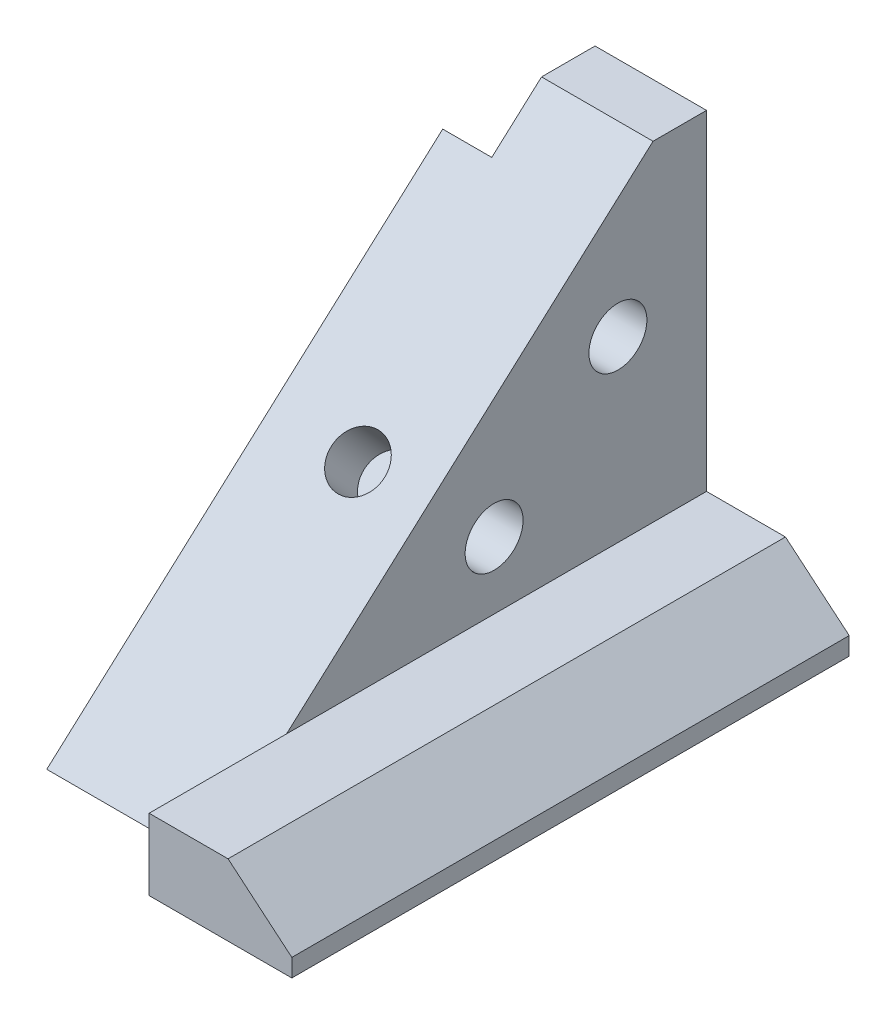
ISO-10303-21;
HEADER;
FILE_DESCRIPTION(('STEP AP214'),'2;1');
FILE_NAME('part.step','',(''),(''),'','','');
FILE_SCHEMA(('AUTOMOTIVE_DESIGN { 1 0 10303 214 1 1 1 1 }'));
ENDSEC;
DATA;
#1=APPLICATION_CONTEXT('core data for automotive mechanical design processes');
#2=APPLICATION_PROTOCOL_DEFINITION('international standard','automotive_design',2000,#1);
#3=PRODUCT_CONTEXT('',#1,'mechanical');
#4=PRODUCT('Part','Part','',(#3));
#5=PRODUCT_RELATED_PRODUCT_CATEGORY('part','',(#4));
#6=PRODUCT_DEFINITION_FORMATION('','',#4);
#7=PRODUCT_DEFINITION_CONTEXT('part definition',#1,'design');
#8=PRODUCT_DEFINITION('design','',#6,#7);
#9=PRODUCT_DEFINITION_SHAPE('','',#8);
#10=(LENGTH_UNIT() NAMED_UNIT(*) SI_UNIT(.MILLI.,.METRE.));
#11=(NAMED_UNIT(*) PLANE_ANGLE_UNIT() SI_UNIT($,.RADIAN.));
#12=(NAMED_UNIT(*) SI_UNIT($,.STERADIAN.) SOLID_ANGLE_UNIT());
#13=UNCERTAINTY_MEASURE_WITH_UNIT(LENGTH_MEASURE(1.E-05),#10,'distance_accuracy_value','');
#14=(GEOMETRIC_REPRESENTATION_CONTEXT(3) GLOBAL_UNCERTAINTY_ASSIGNED_CONTEXT((#13)) GLOBAL_UNIT_ASSIGNED_CONTEXT((#10,
#11,#12)) REPRESENTATION_CONTEXT('',''));
#15=CARTESIAN_POINT('',(0.,0.,0.));
#16=DIRECTION('',(0.,0.,1.));
#17=DIRECTION('',(1.,0.,0.));
#18=AXIS2_PLACEMENT_3D('',#15,#16,#17);
#19=CARTESIAN_POINT('',(0.,0.,125.));
#20=DIRECTION('',(0.,0.,1.));
#21=DIRECTION('',(1.,0.,0.));
#22=AXIS2_PLACEMENT_3D('',#19,#20,#21);
#23=PLANE('',#22);
#24=DIRECTION('',(-1.,0.,0.));
#25=VECTOR('',#24,1.);
#26=CARTESIAN_POINT('',(0.,16.,125.));
#27=LINE('',#26,#25);
#28=CARTESIAN_POINT('',(17.6989568888694,16.,125.));
#29=VERTEX_POINT('',#28);
#30=CARTESIAN_POINT('',(0.,16.,125.));
#31=VERTEX_POINT('',#30);
#32=EDGE_CURVE('E148',#29,#31,#27,.T.);
#33=ORIENTED_EDGE('',*,*,#32,.T.);
#34=DIRECTION('',(0.,1.,0.));
#35=VECTOR('',#34,1.);
#36=CARTESIAN_POINT('',(0.,90.,125.));
#37=LINE('',#36,#35);
#38=CARTESIAN_POINT('',(0.,0.,125.));
#39=VERTEX_POINT('',#38);
#40=EDGE_CURVE('E199',#39,#31,#37,.T.);
#41=ORIENTED_EDGE('',*,*,#40,.F.);
#42=DIRECTION('',(-1.,0.,0.));
#43=VECTOR('',#42,1.);
#44=CARTESIAN_POINT('',(0.,0.,125.));
#45=LINE('',#44,#43);
#46=CARTESIAN_POINT('',(32.,0.,125.));
#47=VERTEX_POINT('',#46);
#48=EDGE_CURVE('E164',#47,#39,#45,.T.);
#49=ORIENTED_EDGE('',*,*,#48,.F.);
#50=DIRECTION('',(0.,1.,0.));
#51=VECTOR('',#50,1.);
#52=CARTESIAN_POINT('',(32.,0.,125.));
#53=LINE('',#52,#51);
#54=CARTESIAN_POINT('',(32.,4.,125.));
#55=VERTEX_POINT('',#54);
#56=EDGE_CURVE('E210',#47,#55,#53,.T.);
#57=ORIENTED_EDGE('',*,*,#56,.T.);
#58=DIRECTION('',(-0.766044443118979,0.642787609686538,0.));
#59=VECTOR('',#58,1.);
#60=CARTESIAN_POINT('',(15.1912446633535,18.1042204035292,125.));
#61=LINE('',#60,#59);
#62=EDGE_CURVE('E206',#55,#29,#61,.T.);
#63=ORIENTED_EDGE('',*,*,#62,.T.);
#64=EDGE_LOOP('',(#33,#41,#49,#57,#63));
#65=FACE_BOUND('',#64,.T.);
#66=ADVANCED_FACE('F41',(#65),#23,.T.);
#67=CARTESIAN_POINT('',(-36.,0.,125.));
#68=DIRECTION('',(-1.,0.,0.));
#69=DIRECTION('',(0.,0.,1.));
#70=AXIS2_PLACEMENT_3D('',#67,#68,#69);
#71=PLANE('',#70);
#72=CARTESIAN_POINT('',(-36.,56.,19.8712945069006));
#73=DIRECTION('',(-1.,0.,0.));
#74=DIRECTION('',(0.,0.,1.));
#75=AXIS2_PLACEMENT_3D('',#72,#73,#74);
#76=CIRCLE('',#75,6.5);
#77=CARTESIAN_POINT('',(-36.,56.,26.3712945069006));
#78=VERTEX_POINT('',#77);
#79=EDGE_CURVE('E407',#78,#78,#76,.T.);
#80=ORIENTED_EDGE('',*,*,#79,.F.);
#81=EDGE_LOOP('',(#80));
#82=FACE_BOUND('',#81,.T.);
#83=CARTESIAN_POINT('',(-36.,31.,47.6366073776308));
#84=DIRECTION('',(-1.,0.,0.));
#85=DIRECTION('',(0.,0.,1.));
#86=AXIS2_PLACEMENT_3D('',#83,#84,#85);
#87=CIRCLE('',#86,6.5);
#88=CARTESIAN_POINT('',(-36.,31.,54.1366073776308));
#89=VERTEX_POINT('',#88);
#90=EDGE_CURVE('E398',#89,#89,#87,.T.);
#91=ORIENTED_EDGE('',*,*,#90,.F.);
#92=EDGE_LOOP('',(#91));
#93=FACE_BOUND('',#92,.T.);
#94=DIRECTION('',(0.,0.707106781186555,0.70710678118654));
#95=VECTOR('',#94,1.);
#96=CARTESIAN_POINT('',(-36.,51.1182175936227,-5.66857897078022));
#97=LINE('',#96,#95);
#98=CARTESIAN_POINT('',(-36.,56.7867965644031,0.));
#99=VERTEX_POINT('',#98);
#100=CARTESIAN_POINT('',(-36.,79.9492667239713,23.1624701595678));
#101=VERTEX_POINT('',#100);
#102=EDGE_CURVE('E124',#99,#101,#97,.T.);
#103=ORIENTED_EDGE('',*,*,#102,.F.);
#104=DIRECTION('',(0.,1.,0.));
#105=VECTOR('',#104,1.);
#106=CARTESIAN_POINT('',(-36.,0.,0.));
#107=LINE('',#106,#105);
#108=CARTESIAN_POINT('',(-36.,0.,0.));
#109=VERTEX_POINT('',#108);
#110=EDGE_CURVE('E133',#109,#99,#107,.T.);
#111=ORIENTED_EDGE('',*,*,#110,.F.);
#112=DIRECTION('',(0.,0.,-1.));
#113=VECTOR('',#112,1.);
#114=CARTESIAN_POINT('',(-36.,0.,125.));
#115=LINE('',#114,#113);
#116=CARTESIAN_POINT('',(-36.,0.,111.955126334629));
#117=VERTEX_POINT('',#116);
#118=EDGE_CURVE('E177',#117,#109,#115,.T.);
#119=ORIENTED_EDGE('',*,*,#118,.F.);
#120=DIRECTION('',(0.,-0.669130606358854,0.743144825477398));
#121=VECTOR('',#120,1.);
#122=CARTESIAN_POINT('',(-36.,90.,12.));
#123=LINE('',#122,#121);
#124=EDGE_CURVE('E130',#101,#117,#123,.T.);
#125=ORIENTED_EDGE('',*,*,#124,.F.);
#126=EDGE_LOOP('',(#103,#111,#119,#125));
#127=FACE_BOUND('',#126,.T.);
#128=ADVANCED_FACE('F43',(#82,#93,#127),#71,.T.);
#129=CARTESIAN_POINT('',(0.,0.,125.));
#130=DIRECTION('',(0.,-1.,0.));
#131=DIRECTION('',(1.,0.,0.));
#132=AXIS2_PLACEMENT_3D('',#129,#130,#131);
#133=PLANE('',#132);
#134=DIRECTION('',(-1.,0.,0.));
#135=VECTOR('',#134,1.);
#136=CARTESIAN_POINT('',(0.,0.,111.955126334629));
#137=LINE('',#136,#135);
#138=CARTESIAN_POINT('',(0.,0.,111.955126334629));
#139=VERTEX_POINT('',#138);
#140=EDGE_CURVE('E145',#139,#117,#137,.T.);
#141=ORIENTED_EDGE('',*,*,#140,.T.);
#142=ORIENTED_EDGE('',*,*,#118,.T.);
#143=DIRECTION('',(-1.,0.,0.));
#144=VECTOR('',#143,1.);
#145=CARTESIAN_POINT('',(0.,0.,0.));
#146=LINE('',#145,#144);
#147=CARTESIAN_POINT('',(32.,0.,0.));
#148=VERTEX_POINT('',#147);
#149=EDGE_CURVE('E142',#148,#109,#146,.T.);
#150=ORIENTED_EDGE('',*,*,#149,.F.);
#151=DIRECTION('',(0.,0.,-1.));
#152=VECTOR('',#151,1.);
#153=CARTESIAN_POINT('',(32.,0.,125.));
#154=LINE('',#153,#152);
#155=EDGE_CURVE('E180',#47,#148,#154,.T.);
#156=ORIENTED_EDGE('',*,*,#155,.F.);
#157=ORIENTED_EDGE('',*,*,#48,.T.);
#158=DIRECTION('',(0.,0.,1.));
#159=VECTOR('',#158,1.);
#160=CARTESIAN_POINT('',(0.,0.,111.955126334629));
#161=LINE('',#160,#159);
#162=EDGE_CURVE('E61',#139,#39,#161,.T.);
#163=ORIENTED_EDGE('',*,*,#162,.F.);
#164=EDGE_LOOP('',(#141,#142,#150,#156,#157,#163));
#165=FACE_BOUND('',#164,.T.);
#166=ADVANCED_FACE('F234',(#165),#133,.T.);
#167=CARTESIAN_POINT('',(32.,0.,125.));
#168=DIRECTION('',(-1.,0.,0.));
#169=DIRECTION('',(0.,0.,1.));
#170=AXIS2_PLACEMENT_3D('',#167,#168,#169);
#171=PLANE('',#170);
#172=DIRECTION('',(0.,1.,0.));
#173=VECTOR('',#172,1.);
#174=CARTESIAN_POINT('',(32.,0.,0.));
#175=LINE('',#174,#173);
#176=CARTESIAN_POINT('',(32.,4.,0.));
#177=VERTEX_POINT('',#176);
#178=EDGE_CURVE('E144',#148,#177,#175,.T.);
#179=ORIENTED_EDGE('',*,*,#178,.T.);
#180=DIRECTION('',(0.,0.,-1.));
#181=VECTOR('',#180,1.);
#182=CARTESIAN_POINT('',(32.,4.,125.));
#183=LINE('',#182,#181);
#184=EDGE_CURVE('E172',#55,#177,#183,.T.);
#185=ORIENTED_EDGE('',*,*,#184,.F.);
#186=ORIENTED_EDGE('',*,*,#56,.F.);
#187=ORIENTED_EDGE('',*,*,#155,.T.);
#188=EDGE_LOOP('',(#179,#185,#186,#187));
#189=FACE_BOUND('',#188,.T.);
#190=ADVANCED_FACE('F235',(#189),#171,.F.);
#191=CARTESIAN_POINT('',(15.1912446633535,18.1042204035292,125.));
#192=DIRECTION('',(-0.642787609686538,-0.766044443118979,0.));
#193=DIRECTION('',(0.766044443118979,-0.642787609686538,0.));
#194=AXIS2_PLACEMENT_3D('',#191,#192,#193);
#195=PLANE('',#194);
#196=DIRECTION('',(-0.766044443118979,0.642787609686538,0.));
#197=VECTOR('',#196,1.);
#198=CARTESIAN_POINT('',(15.1912446633535,18.1042204035292,0.));
#199=LINE('',#198,#197);
#200=CARTESIAN_POINT('',(17.6989568888694,16.,0.));
#201=VERTEX_POINT('',#200);
#202=EDGE_CURVE('E153',#177,#201,#199,.T.);
#203=ORIENTED_EDGE('',*,*,#202,.T.);
#204=DIRECTION('',(0.,0.,-1.));
#205=VECTOR('',#204,1.);
#206=CARTESIAN_POINT('',(17.6989568888694,16.,125.));
#207=LINE('',#206,#205);
#208=EDGE_CURVE('E171',#29,#201,#207,.T.);
#209=ORIENTED_EDGE('',*,*,#208,.F.);
#210=ORIENTED_EDGE('',*,*,#62,.F.);
#211=ORIENTED_EDGE('',*,*,#184,.T.);
#212=EDGE_LOOP('',(#203,#209,#210,#211));
#213=FACE_BOUND('',#212,.T.);
#214=ADVANCED_FACE('F226',(#213),#195,.F.);
#215=CARTESIAN_POINT('',(0.,16.,125.));
#216=DIRECTION('',(0.,-1.,0.));
#217=DIRECTION('',(1.,0.,0.));
#218=AXIS2_PLACEMENT_3D('',#215,#216,#217);
#219=PLANE('',#218);
#220=DIRECTION('',(-1.,0.,0.));
#221=VECTOR('',#220,1.);
#222=CARTESIAN_POINT('',(0.,16.,0.));
#223=LINE('',#222,#221);
#224=CARTESIAN_POINT('',(0.,16.,0.));
#225=VERTEX_POINT('',#224);
#226=EDGE_CURVE('E156',#201,#225,#223,.T.);
#227=ORIENTED_EDGE('',*,*,#226,.T.);
#228=DIRECTION('',(0.,0.,-1.));
#229=VECTOR('',#228,1.);
#230=CARTESIAN_POINT('',(0.,16.,125.));
#231=LINE('',#230,#229);
#232=CARTESIAN_POINT('',(0.,16.,94.1853260973612));
#233=VERTEX_POINT('',#232);
#234=EDGE_CURVE('E166',#233,#225,#231,.T.);
#235=ORIENTED_EDGE('',*,*,#234,.F.);
#236=EDGE_CURVE('E169',#31,#233,#231,.T.);
#237=ORIENTED_EDGE('',*,*,#236,.F.);
#238=ORIENTED_EDGE('',*,*,#32,.F.);
#239=ORIENTED_EDGE('',*,*,#208,.T.);
#240=EDGE_LOOP('',(#227,#235,#237,#238,#239));
#241=FACE_BOUND('',#240,.T.);
#242=ADVANCED_FACE('F220',(#241),#219,.F.);
#243=CARTESIAN_POINT('',(0.,0.,125.));
#244=DIRECTION('',(-1.,0.,0.));
#245=DIRECTION('',(0.,0.,1.));
#246=AXIS2_PLACEMENT_3D('',#243,#244,#245);
#247=PLANE('',#246);
#248=CARTESIAN_POINT('',(0.,56.,19.8712945069006));
#249=DIRECTION('',(-1.,0.,0.));
#250=DIRECTION('',(0.,0.,1.));
#251=AXIS2_PLACEMENT_3D('',#248,#249,#250);
#252=CIRCLE('',#251,6.5);
#253=CARTESIAN_POINT('',(0.,56.,26.3712945069006));
#254=VERTEX_POINT('',#253);
#255=EDGE_CURVE('E136',#254,#254,#252,.T.);
#256=ORIENTED_EDGE('',*,*,#255,.T.);
#257=EDGE_LOOP('',(#256));
#258=FACE_BOUND('',#257,.T.);
#259=CARTESIAN_POINT('',(0.,31.,47.6366073776308));
#260=DIRECTION('',(-1.,0.,0.));
#261=DIRECTION('',(0.,0.,1.));
#262=AXIS2_PLACEMENT_3D('',#259,#260,#261);
#263=CIRCLE('',#262,6.5);
#264=CARTESIAN_POINT('',(0.,31.,54.1366073776308));
#265=VERTEX_POINT('',#264);
#266=EDGE_CURVE('E392',#265,#265,#263,.T.);
#267=ORIENTED_EDGE('',*,*,#266,.T.);
#268=EDGE_LOOP('',(#267));
#269=FACE_BOUND('',#268,.T.);
#270=DIRECTION('',(0.,0.,-1.));
#271=VECTOR('',#270,1.);
#272=CARTESIAN_POINT('',(0.,90.,125.));
#273=LINE('',#272,#271);
#274=CARTESIAN_POINT('',(0.,90.,12.));
#275=VERTEX_POINT('',#274);
#276=CARTESIAN_POINT('',(0.,90.,0.));
#277=VERTEX_POINT('',#276);
#278=EDGE_CURVE('E168',#275,#277,#273,.T.);
#279=ORIENTED_EDGE('',*,*,#278,.F.);
#280=DIRECTION('',(0.,-0.669130606358854,0.743144825477398));
#281=VECTOR('',#280,1.);
#282=CARTESIAN_POINT('',(0.,90.,12.));
#283=LINE('',#282,#281);
#284=EDGE_CURVE('E198',#275,#233,#283,.T.);
#285=ORIENTED_EDGE('',*,*,#284,.T.);
#286=ORIENTED_EDGE('',*,*,#234,.T.);
#287=DIRECTION('',(0.,1.,0.));
#288=VECTOR('',#287,1.);
#289=CARTESIAN_POINT('',(0.,0.,0.));
#290=LINE('',#289,#288);
#291=EDGE_CURVE('E158',#225,#277,#290,.T.);
#292=ORIENTED_EDGE('',*,*,#291,.T.);
#293=EDGE_LOOP('',(#279,#285,#286,#292));
#294=FACE_BOUND('',#293,.T.);
#295=ADVANCED_FACE('F222',(#258,#269,#294),#247,.F.);
#296=CARTESIAN_POINT('',(0.,90.,125.));
#297=DIRECTION('',(0.,-1.,0.));
#298=DIRECTION('',(0.,0.,-1.));
#299=AXIS2_PLACEMENT_3D('',#296,#297,#298);
#300=PLANE('',#299);
#301=DIRECTION('',(-1.,0.,0.));
#302=VECTOR('',#301,1.);
#303=CARTESIAN_POINT('',(0.,90.,0.));
#304=LINE('',#303,#302);
#305=CARTESIAN_POINT('',(-25.,90.,0.));
#306=VERTEX_POINT('',#305);
#307=EDGE_CURVE('E162',#277,#306,#304,.T.);
#308=ORIENTED_EDGE('',*,*,#307,.T.);
#309=DIRECTION('',(0.,0.,1.));
#310=VECTOR('',#309,1.);
#311=CARTESIAN_POINT('',(-25.,90.,125.));
#312=LINE('',#311,#310);
#313=CARTESIAN_POINT('',(-25.,90.,12.));
#314=VERTEX_POINT('',#313);
#315=EDGE_CURVE('E190',#306,#314,#312,.T.);
#316=ORIENTED_EDGE('',*,*,#315,.T.);
#317=DIRECTION('',(-1.,0.,0.));
#318=VECTOR('',#317,1.);
#319=CARTESIAN_POINT('',(0.,90.,12.));
#320=LINE('',#319,#318);
#321=EDGE_CURVE('E150',#275,#314,#320,.T.);
#322=ORIENTED_EDGE('',*,*,#321,.F.);
#323=ORIENTED_EDGE('',*,*,#278,.T.);
#324=EDGE_LOOP('',(#308,#316,#322,#323));
#325=FACE_BOUND('',#324,.T.);
#326=ADVANCED_FACE('F186',(#325),#300,.F.);
#327=CARTESIAN_POINT('',(0.,0.,0.));
#328=DIRECTION('',(0.,0.,1.));
#329=DIRECTION('',(1.,0.,0.));
#330=AXIS2_PLACEMENT_3D('',#327,#328,#329);
#331=PLANE('',#330);
#332=ORIENTED_EDGE('',*,*,#110,.T.);
#333=DIRECTION('',(1.,0.,0.));
#334=VECTOR('',#333,1.);
#335=CARTESIAN_POINT('',(0.,56.7867965644031,0.));
#336=LINE('',#335,#334);
#337=CARTESIAN_POINT('',(-25.,56.7867965644031,0.));
#338=VERTEX_POINT('',#337);
#339=EDGE_CURVE('E119',#99,#338,#336,.T.);
#340=ORIENTED_EDGE('',*,*,#339,.T.);
#341=DIRECTION('',(0.,1.,0.));
#342=VECTOR('',#341,1.);
#343=CARTESIAN_POINT('',(-25.,0.,0.));
#344=LINE('',#343,#342);
#345=EDGE_CURVE('E129',#338,#306,#344,.T.);
#346=ORIENTED_EDGE('',*,*,#345,.T.);
#347=ORIENTED_EDGE('',*,*,#307,.F.);
#348=ORIENTED_EDGE('',*,*,#291,.F.);
#349=ORIENTED_EDGE('',*,*,#226,.F.);
#350=ORIENTED_EDGE('',*,*,#202,.F.);
#351=ORIENTED_EDGE('',*,*,#178,.F.);
#352=ORIENTED_EDGE('',*,*,#149,.T.);
#353=EDGE_LOOP('',(#332,#340,#346,#347,#348,#349,#350,#351,#352));
#354=FACE_BOUND('',#353,.T.);
#355=ADVANCED_FACE('F137',(#354),#331,.F.);
#356=CARTESIAN_POINT('',(0.,0.,0.));
#357=DIRECTION('',(-1.,0.,0.));
#358=DIRECTION('',(0.,0.,1.));
#359=AXIS2_PLACEMENT_3D('',#356,#357,#358);
#360=PLANE('',#359);
#361=ORIENTED_EDGE('',*,*,#236,.T.);
#362=EDGE_CURVE('E200',#233,#139,#283,.T.);
#363=ORIENTED_EDGE('',*,*,#362,.T.);
#364=ORIENTED_EDGE('',*,*,#162,.T.);
#365=ORIENTED_EDGE('',*,*,#40,.T.);
#366=EDGE_LOOP('',(#361,#363,#364,#365));
#367=FACE_BOUND('',#366,.T.);
#368=ADVANCED_FACE('F217',(#367),#360,.T.);
#369=CARTESIAN_POINT('',(0.,90.,12.));
#370=DIRECTION('',(0.,-0.743144825477398,-0.669130606358854));
#371=DIRECTION('',(0.,0.669130606358854,-0.743144825477398));
#372=AXIS2_PLACEMENT_3D('',#369,#370,#371);
#373=PLANE('',#372);
#374=CARTESIAN_POINT('',(-16.,44.8317506260432,62.1644230276428));
#375=DIRECTION('',(0.,0.743144825477398,0.669130606358854));
#376=DIRECTION('',(0.,-0.669130606358854,0.743144825477398));
#377=AXIS2_PLACEMENT_3D('',#374,#375,#376);
#378=CIRCLE('',#377,6.);
#379=CARTESIAN_POINT('',(-16.,40.8169669878901,66.6232919805072));
#380=VERTEX_POINT('',#379);
#381=EDGE_CURVE('E396',#380,#380,#378,.T.);
#382=ORIENTED_EDGE('',*,*,#381,.F.);
#383=EDGE_LOOP('',(#382));
#384=FACE_BOUND('',#383,.T.);
#385=DIRECTION('',(0.,-0.669130606358854,0.743144825477398));
#386=VECTOR('',#385,1.);
#387=CARTESIAN_POINT('',(-25.,90.,12.));
#388=LINE('',#387,#386);
#389=CARTESIAN_POINT('',(-25.,79.9492667239713,23.1624701595678));
#390=VERTEX_POINT('',#389);
#391=EDGE_CURVE('E47',#314,#390,#388,.T.);
#392=ORIENTED_EDGE('',*,*,#391,.T.);
#393=DIRECTION('',(-1.,0.,0.));
#394=VECTOR('',#393,1.);
#395=CARTESIAN_POINT('',(0.,79.9492667239713,23.1624701595678));
#396=LINE('',#395,#394);
#397=EDGE_CURVE('E11',#390,#101,#396,.T.);
#398=ORIENTED_EDGE('',*,*,#397,.T.);
#399=ORIENTED_EDGE('',*,*,#124,.T.);
#400=ORIENTED_EDGE('',*,*,#140,.F.);
#401=ORIENTED_EDGE('',*,*,#362,.F.);
#402=ORIENTED_EDGE('',*,*,#284,.F.);
#403=ORIENTED_EDGE('',*,*,#321,.T.);
#404=EDGE_LOOP('',(#392,#398,#399,#400,#401,#402,#403));
#405=FACE_BOUND('',#404,.T.);
#406=ADVANCED_FACE('F182',(#384,#405),#373,.F.);
#407=CARTESIAN_POINT('',(-25.,51.1182175936227,-5.66857897078022));
#408=DIRECTION('',(0.,-0.70710678118654,0.707106781186555));
#409=DIRECTION('',(0.,-0.707106781186555,-0.70710678118654));
#410=AXIS2_PLACEMENT_3D('',#407,#408,#409);
#411=PLANE('',#410);
#412=ORIENTED_EDGE('',*,*,#102,.T.);
#413=ORIENTED_EDGE('',*,*,#397,.F.);
#414=DIRECTION('',(0.,0.707106781186555,0.70710678118654));
#415=VECTOR('',#414,1.);
#416=CARTESIAN_POINT('',(-25.,51.1182175936227,-5.66857897078022));
#417=LINE('',#416,#415);
#418=EDGE_CURVE('E57',#338,#390,#417,.T.);
#419=ORIENTED_EDGE('',*,*,#418,.F.);
#420=ORIENTED_EDGE('',*,*,#339,.F.);
#421=EDGE_LOOP('',(#412,#413,#419,#420));
#422=FACE_BOUND('',#421,.T.);
#423=ADVANCED_FACE('F125',(#422),#411,.F.);
#424=CARTESIAN_POINT('',(-25.,0.,0.));
#425=DIRECTION('',(1.,0.,0.));
#426=DIRECTION('',(0.,0.,-1.));
#427=AXIS2_PLACEMENT_3D('',#424,#425,#426);
#428=PLANE('',#427);
#429=ORIENTED_EDGE('',*,*,#418,.T.);
#430=ORIENTED_EDGE('',*,*,#391,.F.);
#431=ORIENTED_EDGE('',*,*,#315,.F.);
#432=ORIENTED_EDGE('',*,*,#345,.F.);
#433=EDGE_LOOP('',(#429,#430,#431,#432));
#434=FACE_BOUND('',#433,.T.);
#435=ADVANCED_FACE('F187',(#434),#428,.F.);
#436=CARTESIAN_POINT('',(0.,31.,47.6366073776308));
#437=DIRECTION('',(-1.,0.,0.));
#438=DIRECTION('',(0.,0.,1.));
#439=AXIS2_PLACEMENT_3D('',#436,#437,#438);
#440=CYLINDRICAL_SURFACE('',#439,6.5);
#441=ORIENTED_EDGE('',*,*,#266,.F.);
#442=EDGE_LOOP('',(#441));
#443=FACE_BOUND('',#442,.T.);
#444=ORIENTED_EDGE('',*,*,#90,.T.);
#445=EDGE_LOOP('',(#444));
#446=FACE_BOUND('',#445,.T.);
#447=ADVANCED_FACE('F294',(#443,#446),#440,.F.);
#448=CARTESIAN_POINT('',(0.,56.,19.8712945069006));
#449=DIRECTION('',(-1.,0.,0.));
#450=DIRECTION('',(0.,0.,1.));
#451=AXIS2_PLACEMENT_3D('',#448,#449,#450);
#452=CYLINDRICAL_SURFACE('',#451,6.5);
#453=ORIENTED_EDGE('',*,*,#255,.F.);
#454=EDGE_LOOP('',(#453));
#455=FACE_BOUND('',#454,.T.);
#456=ORIENTED_EDGE('',*,*,#79,.T.);
#457=EDGE_LOOP('',(#456));
#458=FACE_BOUND('',#457,.T.);
#459=ADVANCED_FACE('F299',(#455,#458),#452,.F.);
#460=CARTESIAN_POINT('',(-16.,36.6571575457918,54.8039863576955));
#461=DIRECTION('',(0.,0.743144825477398,0.669130606358854));
#462=DIRECTION('',(0.,-0.669130606358854,0.743144825477398));
#463=AXIS2_PLACEMENT_3D('',#460,#461,#462);
#464=CYLINDRICAL_SURFACE('',#463,6.);
#465=CARTESIAN_POINT('',(-16.,36.6571575457918,54.8039863576955));
#466=DIRECTION('',(0.,0.743144825477398,0.669130606358854));
#467=DIRECTION('',(0.,-0.669130606358854,0.743144825477398));
#468=AXIS2_PLACEMENT_3D('',#465,#466,#467);
#469=CIRCLE('',#468,6.);
#470=CARTESIAN_POINT('',(-16.,32.6423739076387,59.2628553105598));
#471=VERTEX_POINT('',#470);
#472=EDGE_CURVE('E393',#471,#471,#469,.T.);
#473=ORIENTED_EDGE('',*,*,#472,.F.);
#474=EDGE_LOOP('',(#473));
#475=FACE_BOUND('',#474,.T.);
#476=ORIENTED_EDGE('',*,*,#381,.T.);
#477=EDGE_LOOP('',(#476));
#478=FACE_BOUND('',#477,.T.);
#479=ADVANCED_FACE('F308',(#475,#478),#464,.F.);
#480=CARTESIAN_POINT('',(-16.,36.6571575457918,54.8039863576955));
#481=DIRECTION('',(0.,0.743144825477398,0.669130606358854));
#482=DIRECTION('',(0.,-0.669130606358854,0.743144825477398));
#483=AXIS2_PLACEMENT_3D('',#480,#481,#482);
#484=PLANE('',#483);
#485=ORIENTED_EDGE('',*,*,#472,.T.);
#486=EDGE_LOOP('',(#485));
#487=FACE_BOUND('',#486,.T.);
#488=ADVANCED_FACE('F329',(#487),#484,.T.);
#489=CLOSED_SHELL('',(#66,#128,#166,#190,#214,#242,#295,#326,#355,#368,#406,#423,#435,#447,#459,
#479,#488));
#490=MANIFOLD_SOLID_BREP('B2',#489);
#491=ADVANCED_BREP_SHAPE_REPRESENTATION('',(#18,#490),#14);
#492=SHAPE_DEFINITION_REPRESENTATION(#9,#491);
ENDSEC;
END-ISO-10303-21;
